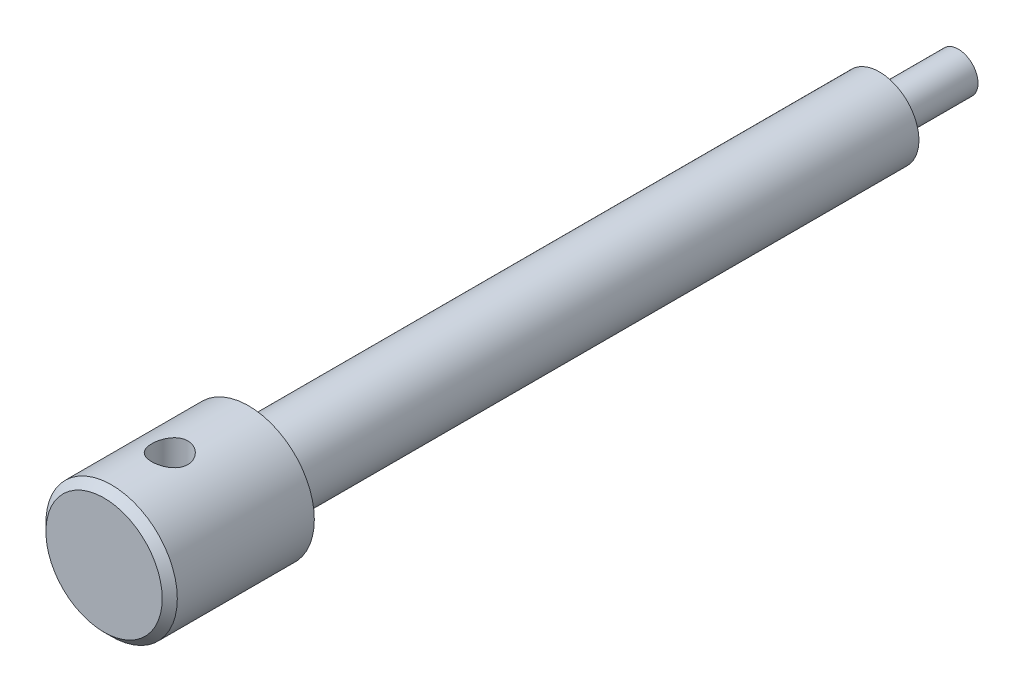
ISO-10303-21;
HEADER;
FILE_DESCRIPTION(('STEP AP214'),'2;1');
FILE_NAME('part.step','',(''),(''),'','','');
FILE_SCHEMA(('AUTOMOTIVE_DESIGN { 1 0 10303 214 1 1 1 1 }'));
ENDSEC;
DATA;
#1=APPLICATION_CONTEXT('core data for automotive mechanical design processes');
#2=APPLICATION_PROTOCOL_DEFINITION('international standard','automotive_design',2000,#1);
#3=PRODUCT_CONTEXT('',#1,'mechanical');
#4=PRODUCT('Part','Part','',(#3));
#5=PRODUCT_RELATED_PRODUCT_CATEGORY('part','',(#4));
#6=PRODUCT_DEFINITION_FORMATION('','',#4);
#7=PRODUCT_DEFINITION_CONTEXT('part definition',#1,'design');
#8=PRODUCT_DEFINITION('design','',#6,#7);
#9=PRODUCT_DEFINITION_SHAPE('','',#8);
#10=(LENGTH_UNIT() NAMED_UNIT(*) SI_UNIT(.MILLI.,.METRE.));
#11=(NAMED_UNIT(*) PLANE_ANGLE_UNIT() SI_UNIT($,.RADIAN.));
#12=(NAMED_UNIT(*) SI_UNIT($,.STERADIAN.) SOLID_ANGLE_UNIT());
#13=UNCERTAINTY_MEASURE_WITH_UNIT(LENGTH_MEASURE(1.E-05),#10,'distance_accuracy_value','');
#14=(GEOMETRIC_REPRESENTATION_CONTEXT(3) GLOBAL_UNCERTAINTY_ASSIGNED_CONTEXT((#13)) GLOBAL_UNIT_ASSIGNED_CONTEXT((#10,
#11,#12)) REPRESENTATION_CONTEXT('',''));
#15=CARTESIAN_POINT('',(0.,0.,0.));
#16=DIRECTION('',(0.,0.,1.));
#17=DIRECTION('',(1.,0.,0.));
#18=AXIS2_PLACEMENT_3D('',#15,#16,#17);
#19=CARTESIAN_POINT('',(0.,0.,22.));
#20=DIRECTION('',(0.,0.,-1.));
#21=DIRECTION('',(-1.,0.,0.));
#22=AXIS2_PLACEMENT_3D('',#19,#20,#21);
#23=CYLINDRICAL_SURFACE('',#22,10.);
#24=CARTESIAN_POINT('',(0.,0.,20.85));
#25=DIRECTION('',(0.,0.,1.));
#26=DIRECTION('',(1.,0.,0.));
#27=AXIS2_PLACEMENT_3D('',#24,#25,#26);
#28=CIRCLE('',#27,10.);
#29=CARTESIAN_POINT('',(10.,0.,20.85));
#30=VERTEX_POINT('',#29);
#31=EDGE_CURVE('E10',#30,#30,#28,.F.);
#32=ORIENTED_EDGE('',*,*,#31,.T.);
#33=EDGE_LOOP('',(#32));
#34=FACE_BOUND('',#33,.T.);
#35=CARTESIAN_POINT('',(0.,-10.,14.75));
#36=CARTESIAN_POINT('',(0.15142288054616,-9.99999790513766,14.7499967849941));
#37=CARTESIAN_POINT('',(0.302879555959281,-9.99652704650773,14.7374514985459));
#38=CARTESIAN_POINT('',(0.601418354260669,-9.9830186270672,14.6876978363444));
#39=CARTESIAN_POINT('',(0.748498536656077,-9.97297819743096,14.6504786858193));
#40=CARTESIAN_POINT('',(1.03393279250043,-9.94743692261125,14.5526875225585));
#41=CARTESIAN_POINT('',(1.17229822737418,-9.93194336798914,14.4921466796217));
#42=CARTESIAN_POINT('',(1.43691255379179,-9.89712668345016,14.3495492113972));
#43=CARTESIAN_POINT('',(1.56316043555,-9.87780323478931,14.2674907951197));
#44=CARTESIAN_POINT('',(1.80305227968481,-9.83687707615023,14.082063533289));
#45=CARTESIAN_POINT('',(1.91635675585361,-9.81523348882719,13.9782645070069));
#46=CARTESIAN_POINT('',(2.12418937034499,-9.77236429681612,13.7532213904992));
#47=CARTESIAN_POINT('',(2.21871492536604,-9.75113874999668,13.6319749040834));
#48=CARTESIAN_POINT('',(2.3879928048007,-9.71108741535023,13.3727300046999));
#49=CARTESIAN_POINT('',(2.46234890182805,-9.69231302357291,13.2344641955079));
#50=CARTESIAN_POINT('',(2.58662289280498,-9.65989315157522,12.9467931991887));
#51=CARTESIAN_POINT('',(2.63654561269354,-9.64624665864575,12.797390218534));
#52=CARTESIAN_POINT('',(2.70934583339765,-9.62605068230367,12.4954588937342));
#53=CARTESIAN_POINT('',(2.73284141478253,-9.61933931887465,12.3430906762779));
#54=CARTESIAN_POINT('',(2.75404817777636,-9.61329031398856,12.0364387731379));
#55=CARTESIAN_POINT('',(2.75176451055439,-9.61395119941996,11.8821554762767));
#56=CARTESIAN_POINT('',(2.72196703105347,-9.62242747025719,11.5809242521359));
#57=CARTESIAN_POINT('',(2.69520726367137,-9.63002901969587,11.4338947522156));
#58=CARTESIAN_POINT('',(2.61842742838165,-9.6511868757216,11.1464974285715));
#59=CARTESIAN_POINT('',(2.56840539656606,-9.66474368507387,11.0061301684078));
#60=CARTESIAN_POINT('',(2.4459209567268,-9.6964683447985,10.7341055891669));
#61=CARTESIAN_POINT('',(2.37319900461751,-9.71468906347739,10.6025715617796));
#62=CARTESIAN_POINT('',(2.20755990360936,-9.75366083636267,10.3533115172166));
#63=CARTESIAN_POINT('',(2.11463855343105,-9.77441241656904,10.2355883804271));
#64=CARTESIAN_POINT('',(1.90740929772698,-9.81699239446062,10.0129908533378));
#65=CARTESIAN_POINT('',(1.79246989633679,-9.83883313993221,9.90870584985344));
#66=CARTESIAN_POINT('',(1.54646529022639,-9.88048509931731,9.7207665138129));
#67=CARTESIAN_POINT('',(1.41539936793062,-9.90029622284757,9.63711309979058));
#68=CARTESIAN_POINT('',(1.13991171237083,-9.93579173537182,9.49252903057962));
#69=CARTESIAN_POINT('',(0.99542816902353,-9.95145560173257,9.43171077717077));
#70=CARTESIAN_POINT('',(0.697756886739508,-9.97674362417589,9.33540050117349));
#71=CARTESIAN_POINT('',(0.544571183725094,-9.98636918666117,9.29990258087253));
#72=CARTESIAN_POINT('',(0.238869177115232,-9.99828101116141,9.25617934751151));
#73=CARTESIAN_POINT('',(0.0864756103297053,-10.0007826748021,9.24715335611134));
#74=CARTESIAN_POINT('',(-0.217649807662516,-9.9987871538593,9.25441110902089));
#75=CARTESIAN_POINT('',(-0.369381730098335,-9.99429074228733,9.27069205791113));
#76=CARTESIAN_POINT('',(-0.664979617013324,-9.97894393202139,9.32744676913747));
#77=CARTESIAN_POINT('',(-0.80893903979837,-9.9682122412504,9.36746883630856));
#78=CARTESIAN_POINT('',(-1.0880827793532,-9.94161719611215,9.47004065820128));
#79=CARTESIAN_POINT('',(-1.22326611385297,-9.92575326850047,9.53259292951927));
#80=CARTESIAN_POINT('',(-1.48409215986275,-9.89015496187791,9.67990036108248));
#81=CARTESIAN_POINT('',(-1.60948250607276,-9.8703479114638,9.76508435615343));
#82=CARTESIAN_POINT('',(-1.84446827852135,-9.82915015297009,9.95470256720286));
#83=CARTESIAN_POINT('',(-1.95406037181207,-9.80775911215361,10.0591408346835));
#84=CARTESIAN_POINT('',(-2.15775026201618,-9.76500318739561,10.2880474208369));
#85=CARTESIAN_POINT('',(-2.25128173000801,-9.74365851048396,10.4130244317764));
#86=CARTESIAN_POINT('',(-2.41606367483463,-9.70411480368907,10.6773558555679));
#87=CARTESIAN_POINT('',(-2.48731502634094,-9.68591565033158,10.816709703729));
#88=CARTESIAN_POINT('',(-2.60498194683926,-9.65493519387949,11.1051872169556));
#89=CARTESIAN_POINT('',(-2.65153712112234,-9.64212352305557,11.2542504979656));
#90=CARTESIAN_POINT('',(-2.71879365333576,-9.62337795912282,11.5585058956763));
#91=CARTESIAN_POINT('',(-2.73950213610858,-9.61744217065576,11.7136963112104));
#92=CARTESIAN_POINT('',(-2.75404886250929,-9.6132857915914,12.0199831380559));
#93=CARTESIAN_POINT('',(-2.7488002394832,-9.614803002412,12.1710332514733));
#94=CARTESIAN_POINT('',(-2.71371466404339,-9.62476380479946,12.4700056933681));
#95=CARTESIAN_POINT('',(-2.6838784224126,-9.63320719614311,12.6179281121346));
#96=CARTESIAN_POINT('',(-2.60100915929162,-9.65590796713359,12.9052149622334));
#97=CARTESIAN_POINT('',(-2.54818121034424,-9.67011387408798,13.044642904425));
#98=CARTESIAN_POINT('',(-2.4209868326845,-9.70273746413612,13.3127643499838));
#99=CARTESIAN_POINT('',(-2.34661683356165,-9.72115584530486,13.4414560693561));
#100=CARTESIAN_POINT('',(-2.17573113118099,-9.76084545820376,13.68878195509));
#101=CARTESIAN_POINT('',(-2.07859788342802,-9.78218767167194,13.8069780917164));
#102=CARTESIAN_POINT('',(-1.86610223089928,-9.82493707924126,14.0256895185393));
#103=CARTESIAN_POINT('',(-1.75073533607713,-9.84634428807069,14.1262004408239));
#104=CARTESIAN_POINT('',(-1.50182041708214,-9.88740569602887,14.308987654299));
#105=CARTESIAN_POINT('',(-1.36791284853874,-9.907007737952,14.390787093516));
#106=CARTESIAN_POINT('',(-1.08770978773099,-9.94166772298476,14.5305864445215));
#107=CARTESIAN_POINT('',(-0.941421808208406,-9.95672839694538,14.5886006666029));
#108=CARTESIAN_POINT('',(-0.66319943123834,-9.97880995779365,14.6721727208583));
#109=CARTESIAN_POINT('',(-0.532391527581486,-9.9866965174671,14.701287579919));
#110=CARTESIAN_POINT('',(-0.267730991455101,-9.9972921723884,14.7402015504145));
#111=CARTESIAN_POINT('',(-0.13387870444774,-10.0000018521471,14.7500028425085));
#112=CARTESIAN_POINT('',(0.,-10.,14.75));
#113=B_SPLINE_CURVE_WITH_KNOTS('',3,(#35,#36,#37,#38,#39,#40,#41,#42,#43,#44,#45,#46,#47,#48,
#49,#50,#51,#52,#53,#54,#55,#56,#57,#58,#59,#60,#61,#62,#63,#64,#65,#66,#67,#68,#69,#70,#71,#72,
#73,#74,#75,#76,#77,#78,#79,#80,#81,#82,#83,#84,#85,#86,#87,#88,#89,#90,#91,#92,#93,#94,#95,#96,
#97,#98,#99,#100,#101,#102,#103,#104,#105,#106,#107,#108,#109,#110,#111,#112),.UNSPECIFIED.,.T.,
.F.,(4,2,2,2,2,2,2,2,2,2,2,2,2,2,2,2,2,2,2,2,2,2,2,2,2,2,2,2,2,2,2,2,2,2,2,2,2,2,4),(0.,
0.45377748539177,0.907753260457005,1.36112438331929,1.81453325397615,2.27794447457157,
2.74141939974404,3.21343018374437,3.68534770125013,4.14598225260575,4.60652476231645,
5.0533402259908,5.50019341874363,5.95235548491221,6.40461168655381,6.87259959045547,
7.34060832576983,7.81089145054107,8.28106499929747,8.73686293716824,9.19261053090921,
9.63995333728771,10.0873461268162,10.5439096300483,11.0005693136824,11.4709880754159,
11.9413883671581,12.4091004005343,12.8766834769387,13.3279371425805,13.7791777637644,
14.2264735227925,14.6738434597267,15.1351456160056,15.5965615457126,16.0686764715747,
16.5405069328285,16.9417541030026,17.3429559665035),.UNSPECIFIED.);
#114=CARTESIAN_POINT('',(0.,-10.,14.75));
#115=VERTEX_POINT('',#114);
#116=EDGE_CURVE('E64',#115,#115,#113,.T.);
#117=ORIENTED_EDGE('',*,*,#116,.T.);
#118=EDGE_LOOP('',(#117));
#119=FACE_BOUND('',#118,.T.);
#120=CARTESIAN_POINT('',(0.,10.,14.75));
#121=CARTESIAN_POINT('',(-0.15142288054616,9.99999790513766,14.7499967849941));
#122=CARTESIAN_POINT('',(-0.302879555959281,9.99652704650773,14.7374514985459));
#123=CARTESIAN_POINT('',(-0.601418354260669,9.9830186270672,14.6876978363444));
#124=CARTESIAN_POINT('',(-0.748498536656077,9.97297819743096,14.6504786858193));
#125=CARTESIAN_POINT('',(-1.03393279250043,9.94743692261125,14.5526875225585));
#126=CARTESIAN_POINT('',(-1.17229822737418,9.93194336798914,14.4921466796217));
#127=CARTESIAN_POINT('',(-1.43691255379179,9.89712668345016,14.3495492113972));
#128=CARTESIAN_POINT('',(-1.56316043555,9.87780323478931,14.2674907951197));
#129=CARTESIAN_POINT('',(-1.80305227968481,9.83687707615023,14.082063533289));
#130=CARTESIAN_POINT('',(-1.91635675585361,9.81523348882719,13.9782645070069));
#131=CARTESIAN_POINT('',(-2.12418937034499,9.77236429681612,13.7532213904992));
#132=CARTESIAN_POINT('',(-2.21871492536604,9.75113874999668,13.6319749040834));
#133=CARTESIAN_POINT('',(-2.3879928048007,9.71108741535023,13.3727300046999));
#134=CARTESIAN_POINT('',(-2.46234890182805,9.69231302357291,13.2344641955079));
#135=CARTESIAN_POINT('',(-2.58662289280498,9.65989315157522,12.9467931991887));
#136=CARTESIAN_POINT('',(-2.63654561269354,9.64624665864575,12.797390218534));
#137=CARTESIAN_POINT('',(-2.70934583339765,9.62605068230367,12.4954588937342));
#138=CARTESIAN_POINT('',(-2.73284141478253,9.61933931887465,12.3430906762779));
#139=CARTESIAN_POINT('',(-2.75404817777636,9.61329031398856,12.0364387731379));
#140=CARTESIAN_POINT('',(-2.75176451055439,9.61395119941996,11.8821554762767));
#141=CARTESIAN_POINT('',(-2.72196703105347,9.62242747025719,11.5809242521359));
#142=CARTESIAN_POINT('',(-2.69520726367137,9.63002901969587,11.4338947522156));
#143=CARTESIAN_POINT('',(-2.61842742838165,9.6511868757216,11.1464974285715));
#144=CARTESIAN_POINT('',(-2.56840539656606,9.66474368507387,11.0061301684078));
#145=CARTESIAN_POINT('',(-2.4459209567268,9.6964683447985,10.7341055891669));
#146=CARTESIAN_POINT('',(-2.37319900461751,9.71468906347739,10.6025715617796));
#147=CARTESIAN_POINT('',(-2.20755990360936,9.75366083636267,10.3533115172166));
#148=CARTESIAN_POINT('',(-2.11463855343105,9.77441241656904,10.2355883804271));
#149=CARTESIAN_POINT('',(-1.90740929772698,9.81699239446062,10.0129908533378));
#150=CARTESIAN_POINT('',(-1.79246989633679,9.83883313993221,9.90870584985344));
#151=CARTESIAN_POINT('',(-1.54646529022639,9.88048509931731,9.7207665138129));
#152=CARTESIAN_POINT('',(-1.41539936793062,9.90029622284757,9.63711309979058));
#153=CARTESIAN_POINT('',(-1.13991171237083,9.93579173537182,9.49252903057962));
#154=CARTESIAN_POINT('',(-0.99542816902353,9.95145560173257,9.43171077717077));
#155=CARTESIAN_POINT('',(-0.697756886739508,9.97674362417589,9.33540050117349));
#156=CARTESIAN_POINT('',(-0.544571183725094,9.98636918666117,9.29990258087253));
#157=CARTESIAN_POINT('',(-0.238869177115232,9.99828101116141,9.25617934751151));
#158=CARTESIAN_POINT('',(-0.0864756103297053,10.0007826748021,9.24715335611134));
#159=CARTESIAN_POINT('',(0.217649807662516,9.9987871538593,9.25441110902089));
#160=CARTESIAN_POINT('',(0.369381730098335,9.99429074228733,9.27069205791113));
#161=CARTESIAN_POINT('',(0.664979617013324,9.97894393202139,9.32744676913747));
#162=CARTESIAN_POINT('',(0.80893903979837,9.9682122412504,9.36746883630856));
#163=CARTESIAN_POINT('',(1.0880827793532,9.94161719611215,9.47004065820128));
#164=CARTESIAN_POINT('',(1.22326611385297,9.92575326850047,9.53259292951927));
#165=CARTESIAN_POINT('',(1.48409215986275,9.89015496187791,9.67990036108248));
#166=CARTESIAN_POINT('',(1.60948250607276,9.8703479114638,9.76508435615343));
#167=CARTESIAN_POINT('',(1.84446827852135,9.82915015297009,9.95470256720286));
#168=CARTESIAN_POINT('',(1.95406037181207,9.80775911215361,10.0591408346835));
#169=CARTESIAN_POINT('',(2.15775026201618,9.76500318739561,10.2880474208369));
#170=CARTESIAN_POINT('',(2.25128173000801,9.74365851048396,10.4130244317764));
#171=CARTESIAN_POINT('',(2.41606367483463,9.70411480368907,10.6773558555679));
#172=CARTESIAN_POINT('',(2.48731502634094,9.68591565033158,10.816709703729));
#173=CARTESIAN_POINT('',(2.60498194683926,9.65493519387949,11.1051872169556));
#174=CARTESIAN_POINT('',(2.65153712112234,9.64212352305557,11.2542504979656));
#175=CARTESIAN_POINT('',(2.71879365333576,9.62337795912282,11.5585058956763));
#176=CARTESIAN_POINT('',(2.73950213610858,9.61744217065576,11.7136963112104));
#177=CARTESIAN_POINT('',(2.75404886250929,9.6132857915914,12.0199831380559));
#178=CARTESIAN_POINT('',(2.7488002394832,9.614803002412,12.1710332514733));
#179=CARTESIAN_POINT('',(2.71371466404339,9.62476380479946,12.4700056933681));
#180=CARTESIAN_POINT('',(2.6838784224126,9.63320719614311,12.6179281121346));
#181=CARTESIAN_POINT('',(2.60100915929162,9.65590796713359,12.9052149622334));
#182=CARTESIAN_POINT('',(2.54818121034424,9.67011387408798,13.044642904425));
#183=CARTESIAN_POINT('',(2.4209868326845,9.70273746413612,13.3127643499838));
#184=CARTESIAN_POINT('',(2.34661683356165,9.72115584530486,13.4414560693561));
#185=CARTESIAN_POINT('',(2.17573113118099,9.76084545820376,13.68878195509));
#186=CARTESIAN_POINT('',(2.07859788342802,9.78218767167194,13.8069780917164));
#187=CARTESIAN_POINT('',(1.86610223089928,9.82493707924126,14.0256895185393));
#188=CARTESIAN_POINT('',(1.75073533607713,9.84634428807069,14.1262004408239));
#189=CARTESIAN_POINT('',(1.50182041708214,9.88740569602887,14.308987654299));
#190=CARTESIAN_POINT('',(1.36791284853874,9.907007737952,14.390787093516));
#191=CARTESIAN_POINT('',(1.08770978773099,9.94166772298476,14.5305864445215));
#192=CARTESIAN_POINT('',(0.941421808208406,9.95672839694538,14.5886006666029));
#193=CARTESIAN_POINT('',(0.66319943123834,9.97880995779365,14.6721727208583));
#194=CARTESIAN_POINT('',(0.532391527581486,9.9866965174671,14.701287579919));
#195=CARTESIAN_POINT('',(0.267730991455101,9.9972921723884,14.7402015504145));
#196=CARTESIAN_POINT('',(0.13387870444774,10.0000018521471,14.7500028425085));
#197=CARTESIAN_POINT('',(0.,10.,14.75));
#198=B_SPLINE_CURVE_WITH_KNOTS('',3,(#120,#121,#122,#123,#124,#125,#126,#127,#128,#129,#130,
#131,#132,#133,#134,#135,#136,#137,#138,#139,#140,#141,#142,#143,#144,#145,#146,#147,#148,#149,
#150,#151,#152,#153,#154,#155,#156,#157,#158,#159,#160,#161,#162,#163,#164,#165,#166,#167,#168,
#169,#170,#171,#172,#173,#174,#175,#176,#177,#178,#179,#180,#181,#182,#183,#184,#185,#186,#187,
#188,#189,#190,#191,#192,#193,#194,#195,#196,#197),.UNSPECIFIED.,.T.,.F.,(4,2,2,2,2,2,2,2,2,2,2,
2,2,2,2,2,2,2,2,2,2,2,2,2,2,2,2,2,2,2,2,2,2,2,2,2,2,2,4),(0.,0.45377748539177,0.907753260457005,
1.36112438331929,1.81453325397615,2.27794447457157,2.74141939974404,3.21343018374437,
3.68534770125013,4.14598225260575,4.60652476231645,5.0533402259908,5.50019341874363,
5.95235548491221,6.40461168655381,6.87259959045547,7.34060832576983,7.81089145054107,
8.28106499929747,8.73686293716824,9.19261053090921,9.63995333728771,10.0873461268162,
10.5439096300483,11.0005693136824,11.4709880754159,11.9413883671581,12.4091004005343,
12.8766834769387,13.3279371425805,13.7791777637644,14.2264735227925,14.6738434597267,
15.1351456160056,15.5965615457126,16.0686764715747,16.5405069328285,16.9417541030026,
17.3429559665035),.UNSPECIFIED.);
#199=CARTESIAN_POINT('',(0.,10.,14.75));
#200=VERTEX_POINT('',#199);
#201=EDGE_CURVE('E75',#200,#200,#198,.T.);
#202=ORIENTED_EDGE('',*,*,#201,.T.);
#203=EDGE_LOOP('',(#202));
#204=FACE_BOUND('',#203,.T.);
#205=CARTESIAN_POINT('',(0.,0.,0.));
#206=DIRECTION('',(0.,0.,1.));
#207=DIRECTION('',(1.,0.,0.));
#208=AXIS2_PLACEMENT_3D('',#205,#206,#207);
#209=CIRCLE('',#208,10.);
#210=CARTESIAN_POINT('',(10.,0.,0.));
#211=VERTEX_POINT('',#210);
#212=EDGE_CURVE('E125',#211,#211,#209,.T.);
#213=ORIENTED_EDGE('',*,*,#212,.T.);
#214=EDGE_LOOP('',(#213));
#215=FACE_BOUND('',#214,.T.);
#216=ADVANCED_FACE('F44',(#34,#119,#204,#215),#23,.T.);
#217=CARTESIAN_POINT('',(0.,0.,22.));
#218=DIRECTION('',(0.,0.,1.));
#219=DIRECTION('',(1.,0.,0.));
#220=AXIS2_PLACEMENT_3D('',#217,#218,#219);
#221=PLANE('',#220);
#222=CARTESIAN_POINT('',(0.,0.,22.));
#223=DIRECTION('',(0.,0.,1.));
#224=DIRECTION('',(1.,0.,0.));
#225=AXIS2_PLACEMENT_3D('',#222,#223,#224);
#226=CIRCLE('',#225,8.85);
#227=CARTESIAN_POINT('',(8.85,0.,22.));
#228=VERTEX_POINT('',#227);
#229=EDGE_CURVE('E52',#228,#228,#226,.T.);
#230=ORIENTED_EDGE('',*,*,#229,.T.);
#231=EDGE_LOOP('',(#230));
#232=FACE_BOUND('',#231,.T.);
#233=ADVANCED_FACE('F105',(#232),#221,.T.);
#234=CARTESIAN_POINT('',(0.,0.,0.));
#235=DIRECTION('',(0.,0.,1.));
#236=DIRECTION('',(1.,0.,0.));
#237=AXIS2_PLACEMENT_3D('',#234,#235,#236);
#238=PLANE('',#237);
#239=CARTESIAN_POINT('',(0.,0.,0.));
#240=DIRECTION('',(0.,0.,-1.));
#241=DIRECTION('',(-1.,0.,0.));
#242=AXIS2_PLACEMENT_3D('',#239,#240,#241);
#243=CIRCLE('',#242,6.);
#244=CARTESIAN_POINT('',(-6.,0.,0.));
#245=VERTEX_POINT('',#244);
#246=EDGE_CURVE('E63',#245,#245,#243,.T.);
#247=ORIENTED_EDGE('',*,*,#246,.F.);
#248=EDGE_LOOP('',(#247));
#249=FACE_BOUND('',#248,.T.);
#250=ORIENTED_EDGE('',*,*,#212,.F.);
#251=EDGE_LOOP('',(#250));
#252=FACE_BOUND('',#251,.T.);
#253=ADVANCED_FACE('F99',(#249,#252),#238,.F.);
#254=CARTESIAN_POINT('',(0.,0.,-96.));
#255=DIRECTION('',(0.,0.,1.));
#256=DIRECTION('',(1.,0.,0.));
#257=AXIS2_PLACEMENT_3D('',#254,#255,#256);
#258=CYLINDRICAL_SURFACE('',#257,6.);
#259=CARTESIAN_POINT('',(0.,0.,-96.));
#260=DIRECTION('',(0.,0.,-1.));
#261=DIRECTION('',(-1.,0.,0.));
#262=AXIS2_PLACEMENT_3D('',#259,#260,#261);
#263=CIRCLE('',#262,6.);
#264=CARTESIAN_POINT('',(-6.,0.,-96.));
#265=VERTEX_POINT('',#264);
#266=EDGE_CURVE('E122',#265,#265,#263,.T.);
#267=ORIENTED_EDGE('',*,*,#266,.F.);
#268=EDGE_LOOP('',(#267));
#269=FACE_BOUND('',#268,.T.);
#270=ORIENTED_EDGE('',*,*,#246,.T.);
#271=EDGE_LOOP('',(#270));
#272=FACE_BOUND('',#271,.T.);
#273=ADVANCED_FACE('F96',(#269,#272),#258,.T.);
#274=CARTESIAN_POINT('',(0.,0.,-96.));
#275=DIRECTION('',(0.,0.,-1.));
#276=DIRECTION('',(-1.,0.,0.));
#277=AXIS2_PLACEMENT_3D('',#274,#275,#276);
#278=PLANE('',#277);
#279=CARTESIAN_POINT('',(0.,0.,-96.));
#280=DIRECTION('',(0.,0.,-1.));
#281=DIRECTION('',(-1.,0.,0.));
#282=AXIS2_PLACEMENT_3D('',#279,#280,#281);
#283=CIRCLE('',#282,3.);
#284=CARTESIAN_POINT('',(-3.,0.,-96.));
#285=VERTEX_POINT('',#284);
#286=EDGE_CURVE('E60',#285,#285,#283,.T.);
#287=ORIENTED_EDGE('',*,*,#286,.F.);
#288=EDGE_LOOP('',(#287));
#289=FACE_BOUND('',#288,.T.);
#290=ORIENTED_EDGE('',*,*,#266,.T.);
#291=EDGE_LOOP('',(#290));
#292=FACE_BOUND('',#291,.T.);
#293=ADVANCED_FACE('F95',(#289,#292),#278,.T.);
#294=CARTESIAN_POINT('',(0.,0.,-108.));
#295=DIRECTION('',(0.,0.,1.));
#296=DIRECTION('',(1.,0.,0.));
#297=AXIS2_PLACEMENT_3D('',#294,#295,#296);
#298=CYLINDRICAL_SURFACE('',#297,3.);
#299=CARTESIAN_POINT('',(0.,0.,-108.));
#300=DIRECTION('',(0.,0.,-1.));
#301=DIRECTION('',(-1.,0.,0.));
#302=AXIS2_PLACEMENT_3D('',#299,#300,#301);
#303=CIRCLE('',#302,3.);
#304=CARTESIAN_POINT('',(-3.,0.,-108.));
#305=VERTEX_POINT('',#304);
#306=EDGE_CURVE('E72',#305,#305,#303,.T.);
#307=ORIENTED_EDGE('',*,*,#306,.F.);
#308=EDGE_LOOP('',(#307));
#309=FACE_BOUND('',#308,.T.);
#310=ORIENTED_EDGE('',*,*,#286,.T.);
#311=EDGE_LOOP('',(#310));
#312=FACE_BOUND('',#311,.T.);
#313=ADVANCED_FACE('F86',(#309,#312),#298,.T.);
#314=CARTESIAN_POINT('',(0.,0.,-108.));
#315=DIRECTION('',(0.,0.,-1.));
#316=DIRECTION('',(-1.,0.,0.));
#317=AXIS2_PLACEMENT_3D('',#314,#315,#316);
#318=PLANE('',#317);
#319=ORIENTED_EDGE('',*,*,#306,.T.);
#320=EDGE_LOOP('',(#319));
#321=FACE_BOUND('',#320,.T.);
#322=ADVANCED_FACE('F82',(#321),#318,.T.);
#323=CARTESIAN_POINT('',(0.,-12.,12.));
#324=DIRECTION('',(0.,1.,0.));
#325=DIRECTION('',(0.,0.,1.));
#326=AXIS2_PLACEMENT_3D('',#323,#324,#325);
#327=CYLINDRICAL_SURFACE('',#326,2.75);
#328=ORIENTED_EDGE('',*,*,#201,.F.);
#329=EDGE_LOOP('',(#328));
#330=FACE_BOUND('',#329,.T.);
#331=ORIENTED_EDGE('',*,*,#116,.F.);
#332=EDGE_LOOP('',(#331));
#333=FACE_BOUND('',#332,.T.);
#334=ADVANCED_FACE('F79',(#330,#333),#327,.F.);
#335=CARTESIAN_POINT('',(0.,0.,22.));
#336=DIRECTION('',(0.,0.,-1.));
#337=DIRECTION('',(-1.,0.,0.));
#338=AXIS2_PLACEMENT_3D('',#335,#336,#337);
#339=CONICAL_SURFACE('',#338,8.85,0.785398163397443);
#340=ORIENTED_EDGE('',*,*,#31,.F.);
#341=EDGE_LOOP('',(#340));
#342=FACE_BOUND('',#341,.T.);
#343=ORIENTED_EDGE('',*,*,#229,.F.);
#344=EDGE_LOOP('',(#343));
#345=FACE_BOUND('',#344,.T.);
#346=ADVANCED_FACE('F48',(#342,#345),#339,.T.);
#347=CLOSED_SHELL('',(#216,#233,#253,#273,#293,#313,#322,#334,#346));
#348=MANIFOLD_SOLID_BREP('B2',#347);
#349=ADVANCED_BREP_SHAPE_REPRESENTATION('',(#18,#348),#14);
#350=SHAPE_DEFINITION_REPRESENTATION(#9,#349);
ENDSEC;
END-ISO-10303-21;
